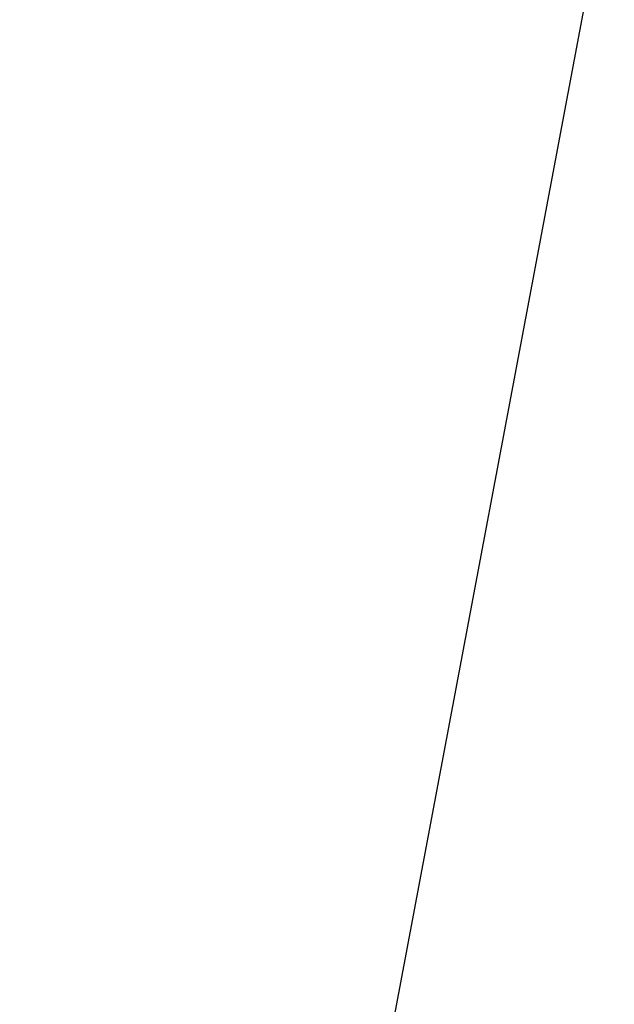
# Model space of a CAD drawing. Units: inches. Extents: x 3590 to 5167, y 65 to 1917.
# Tile 83 of 100: x 5051.4139 to 5051.5399, y 1788.6144 to 1788.8231. Entities that reach past the tile are written whole.
import ezdxf

# ---------------------------------------------------------------- set-up
doc = ezdxf.new("R2010")
doc.units = ezdxf.units.IN
for name, color, linetype, lineweight in [('A-ANNO-DIMS', 2, 'Continuous', 18), ('A-FLOR-PATT', 8, 'Continuous', 13), ('L-PLNT', 94, 'Continuous', 18)]:
    doc.layers.add(name, color=color, linetype=linetype, lineweight=lineweight)
doc.layers.add('DIENHOA', color=3, linetype='Continuous')
doc.styles.get("Standard").update_dxf_attribs({"font": 'arial.ttf'})
doc.dimstyles.new('ISO-25', dxfattribs={"dimtxt": 9, "dimasz": 2.5, "dimexe": 1.25, "dimexo": 0.625, "dimtad": 1, "dimdec": 1, "dimlunit": 3, "dimtxsty": 'Standard', "dimcen": 2.5, "dimadec": 0, "dimazin": 0, "dimtfac": 1, "dimtdec": 1, "dimtmove": 0, "dimatfit": 3, "dimfxl": 1, "dimarcsym": 0})

# ---------------------------------------------------------------- blocks, each defined once
blk = doc.blocks.new('Cay03_mb')
at = {"layer": 'DIENHOA'}
blk.add_lwpolyline([(87.9153, 628.5249), (75.4561, 544.1788), (61.2665, 461.1547), (46.1288, 379.1401), (30.8256, 297.8222), (16.1394, 216.8885), (2.8527, 136.0262), (-8.252, 54.9228), (-16.3923, -26.7346)], dxfattribs=at)
blk = doc.blocks.new('*D323')
at = {"layer": 'A-ANNO-DIMS', "color": 0, "lineweight": -2, "transparency": 16777216}
for p, q in [((5069.17227, 1795.21603), (5069.17227, 1874.95034)), ((5065.43703, 1795.21603), (5070.42227, 1795.21603)), ((5069.17227, 1769.30924), (5069.17227, 1792.71603)), ((5065.43703, 1766.80924), (5070.42227, 1766.80924))]:
    blk.add_line(p, q, dxfattribs=at)
at = {"layer": 'A-ANNO-DIMS', "color": 0, "transparency": 16777216}
for points in [[(5068.75561, 1792.71603), (5069.58894, 1792.71603), (5069.17227, 1795.21603)], [(5068.75561, 1769.30924), (5069.58894, 1769.30924), (5069.17227, 1766.80924)]]:
    blk.add_solid(points, dxfattribs=at)
at = {"layer": 'Defpoints', "color": 0, "transparency": 16777216}
for p in [(5064.81203, 1795.21603), (5069.17227, 1795.21603), (5064.81203, 1766.80924)]:
    blk.add_point(p, dxfattribs=at)
at = {"layer": 'A-ANNO-DIMS', "color": 0, "transparency": 16777216, "insert": (5063.89379, 1836.33318), "char_height": 9, "attachment_point": 5, "rotation": 90}
blk.add_mtext('2\'-4 1/2" TYP.', dxfattribs=at)

msp = doc.modelspace()

# ---------------------------------------------------------------- hatches: boundary and pattern name
at = {"layer": 'A-FLOR-PATT', "transparency": 33554687}
h = msp.add_hatch(dxfattribs=at)
h.set_pattern_fill('AR-HBONE', color=256, scale=0.2)
h.set_pattern_definition([(45, (-588.972, 0), (0, 28.73682), [60.96, -20.32]), (135, (-574.604, 14.368), (3e-15, 28.73682), [60.96, -20.32])])
h.paths.add_polyline_path([(5071.27403, 1796.99898), (4933.27403, 1796.99898), (4933.27403, 1753.99898), (4962.77403, 1753.99898, -0.414214), (4928.77403, 1719.99898), (4933.27403, 1718.99898), (4933.27403, 1334.99898), (5071.27403, 1334.99898)])
h.paths.add_polyline_path([(4951.78002, 1521.0767), (4951.7151, 1521.0404), (4951.56345, 1520.89532)], flags=16)
h.paths.add_polyline_path([(4952.267, 1521.37645), (4952.1977, 1521.37111), (4952.19823, 1521.35558)], flags=0)
h.paths.add_polyline_path([(4967.05076, 1529.72832), (4965.23122, 1528.69444), (4963.41109, 1527.71401), (4961.75649, 1526.85081), (4963.58887, 1527.44938), (4964.03555, 1527.47802), (4962.9755, 1527.24902), (4961.76022, 1526.85203), (4959.79219, 1525.83406), (4958.00498, 1524.89483), (4956.24031, 1523.92961), (4954.50395, 1522.91854), (4954.1294, 1522.68163), (4953.36051, 1521.99688), (4953.36558, 1521.99754), (4953.605, 1522.06367), (4955.10605, 1522.76083), (4956.92108, 1523.43405), (4958.67784, 1523.91513), (4960.35834, 1524.20036), (4961.94456, 1524.28606), (4964.17144, 1524.10849), (4965.95752, 1523.30903), (4963.86273, 1522.97565), (4965.18742, 1522.49898), (4963.36614, 1522.49715), (4961.54526, 1522.48682), (4959.76359, 1522.46077), (4958.30414, 1522.4188), (4957.97356, 1522.38829), (4956.30692, 1522.2324), (4954.71821, 1522.07143), (4953.25077, 1521.89915), (4953.52509, 1521.62277), (4954.33087, 1521.37883), (4956.24263, 1521.22987), (4958.03913, 1520.92952), (4959.68424, 1520.48339), (4961.16007, 1519.89569), (4963.10699, 1518.80022), (4964.39286, 1517.32518), (4962.97306, 1517.72596), (4964.55841, 1516.66059), (4965.40664, 1515.70779), (4963.50733, 1516.32179), (4961.67995, 1517.0051), (4959.93478, 1517.74489), (4958.2821, 1518.52833), (4956.73216, 1519.34257), (4955.29527, 1520.17478), (4954.67155, 1520.57237), (4954.51279, 1520.6271), (4955.65848, 1519.31837), (4956.70263, 1517.98232), (4957.64403, 1516.64663), (4958.48545, 1515.33439), (4959.54998, 1513.52398), (4960.43768, 1511.76936), (4958.84107, 1513.6196), (4957.45175, 1515.3249), (4955.8186, 1517.45855), (4956.66537, 1515.44764), (4957.11109, 1513.92292), (4957.44681, 1511.71434), (4957.07641, 1509.79288), (4956.53757, 1511.1103), (4955.99231, 1512.56892), (4955.44448, 1514.12509), (4954.89794, 1515.73518), (4954.35653, 1517.35553), (4953.82412, 1518.94251), (4953.30455, 1520.45247), (4953.06452, 1521.11563), (4952.97143, 1521.14607), (4952.94932, 1521.08646), (4952.72981, 1520.19905), (4953.3698, 1518.02364), (4953.75708, 1516.37279), (4954.05124, 1514.76538), (4954.26449, 1513.22121), (4954.47124, 1511.13121), (4954.4971, 1510.40174), (4954.40903, 1511.76006), (4954.26449, 1513.22121), (4954.05124, 1514.76538), (4953.75708, 1516.37279), (4953.3698, 1518.02364), (4952.87718, 1519.69813), (4952.7161, 1520.1412), (4952.53301, 1519.05871), (4952.37428, 1517.78881), (4952.21925, 1516.31167), (4952.04598, 1514.59986), (4951.83253, 1512.62598), (4951.55697, 1510.36259), (4951.20331, 1512.16818), (4950.85168, 1514.33931), (4950.98529, 1516.37594), (4951.6596, 1518.28625), (4952.59261, 1520.48085), (4952.35664, 1521.1299), (4951.85502, 1520.32753), (4950.83901, 1518.90828), (4949.77675, 1517.58658), (4948.91554, 1516.61731), (4948.11099, 1515.2561), (4947.0891, 1513.55389), (4945.88937, 1511.61495), (4946.32587, 1513.40232), (4946.5624, 1514.24913), (4945.52771, 1513.32668), (4944.58105, 1512.53126), (4946.01774, 1514.50825), (4947.2044, 1516.04763), (4947.89331, 1517.31331), (4949.30686, 1518.76446), (4950.41417, 1519.76716), (4950.45131, 1519.80628), (4952.267, 1521.37645), (4951.64457, 1521.49317), (4950.40371, 1521.17954), (4948.04447, 1520.35868), (4946.11863, 1519.45198), (4944.57182, 1518.47484), (4943.34962, 1517.44265), (4941.99695, 1515.91971), (4941.66146, 1515.27475), (4942.81332, 1516.98973), (4944.57182, 1518.47484), (4946.11863, 1519.45198), (4948.04447, 1520.35868), (4950.40371, 1521.17954), (4951.64457, 1521.49317), (4949.64678, 1521.86781), (4948.59979, 1521.75633), (4947.12629, 1521.5699), (4945.42015, 1521.34763), (4943.44969, 1521.10462), (4941.18319, 1520.85596), (4942.86028, 1521.61265), (4943.87308, 1522.03014), (4942.95216, 1521.9093), (4941.40968, 1521.48512), (4939.54287, 1520.67019), (4938.96775, 1520.2255), (4940.73284, 1521.29899), (4942.95216, 1521.9093), (4943.70184, 1522.00767), (4945.89419, 1522.69998), (4947.56488, 1522.71399), (4948.92086, 1522.56573), (4951.13144, 1522.18271), (4950.97062, 1522.2969), (4948.12924, 1523.00563), (4946.03496, 1523.70671), (4944.23235, 1524.52143), (4942.70692, 1525.46111), (4941.44419, 1526.53707), (4940.42968, 1527.76062), (4939.6489, 1529.14306), (4941.42091, 1528.12232), (4943.14742, 1527.13248), (4944.84093, 1526.17457), (4946.51394, 1525.24959), (4948.17893, 1524.35855), (4948.36457, 1524.26336), (4946.47531, 1526.04459), (4945.18083, 1527.54042), (4944.19039, 1529.03339), (4943.49559, 1530.53985), (4943.27808, 1531.3597), (4942.49849, 1531.91903), (4943.11353, 1531.76249), (4942.95927, 1533.6586), (4944.13953, 1531.9886), (4944.61171, 1531.32339), (4946.20163, 1530.46341), (4947.48567, 1529.50925), (4948.79027, 1528.22649), (4950.36754, 1526.23746), (4949.48547, 1528.15549), (4948.85128, 1530.12254), (4948.49054, 1532.04127), (4948.38105, 1533.91822), (4948.50062, 1535.7599), (4948.82704, 1537.57284), (4949.41803, 1535.56526), (4949.95684, 1533.56932), (4950.46414, 1531.5861), (4950.96058, 1529.6167), (4951.3911, 1527.95448), (4951.72352, 1530.68689), (4952.20106, 1532.57994), (4952.88914, 1534.32964), (4953.77035, 1535.95123), (4954.82726, 1537.45995), (4954.52145, 1535.38966), (4954.27314, 1533.93684), (4955.57999, 1535.6627), (4956.74758, 1536.73859), (4956.15852, 1534.78029), (4955.58917, 1532.87334), (4955.04336, 1531.00581), (4954.52493, 1529.16576), (4954.03771, 1527.34127), (4953.63833, 1525.73298), (4953.61143, 1525.58564), (4953.39805, 1524.16565), (4953.38219, 1524.00887), (4954.06955, 1525.47563), (4954.91212, 1527.02173), (4956.13627, 1528.89351), (4957.84668, 1530.57701), (4959.37601, 1531.54014), (4958.25596, 1530.10398), (4957.14284, 1528.66291), (4956.06626, 1527.24305), (4955.05579, 1525.87054), (4954.14104, 1524.57149), (4953.35159, 1523.37204), (4953.31079, 1523.30299), (4953.27253, 1522.92478), (4953.26102, 1522.38213), (4954.1031, 1523.37273), (4954.63005, 1524.28376), (4955.96149, 1526.35767), (4957.23002, 1528.12969), (4958.42057, 1529.60864), (4960.03671, 1531.36792), (4961.3736, 1532.3752), (4962.1015, 1532.77), (4961.06994, 1531.06113), (4959.98733, 1529.43811), (4958.86851, 1527.90803), (4958.15046, 1527.00742), (4959.80291, 1528.00314), (4961.58854, 1528.79257), (4963.39087, 1529.32783), (4965.21118, 1529.63205)], flags=16)
h.paths.add_polyline_path([(4962.94387, 1523.18187), (4961.10714, 1523.42192), (4960.39205, 1523.36158), (4962.34964, 1523.33061)], flags=0)
h.paths.add_polyline_path([(5049.54129, 1584.55089), (5049.47636, 1584.51458), (5049.32471, 1584.3695)], flags=16)
h.paths.add_polyline_path([(5050.02827, 1584.85063), (5049.95897, 1584.84529), (5049.95949, 1584.82976)], flags=0)
h.paths.add_polyline_path([(5042.33308, 1581.94902), (5043.8799, 1582.92616), (5045.80573, 1583.83286), (5048.16498, 1584.65372), (5049.40583, 1584.96736), (5047.40804, 1585.34199), (5046.36106, 1585.23052), (5044.88755, 1585.04408), (5043.18142, 1584.82181), (5041.21095, 1584.5788), (5038.94446, 1584.33014), (5040.62155, 1585.08683), (5041.63434, 1585.50432), (5040.71343, 1585.38348), (5039.17095, 1584.9593), (5037.30414, 1584.14438), (5036.72901, 1583.69969), (5038.4941, 1584.77317), (5040.71343, 1585.38348), (5041.4631, 1585.48185), (5043.65545, 1586.17416), (5045.32615, 1586.18818), (5046.68212, 1586.03992), (5048.8927, 1585.6569), (5048.73188, 1585.77108), (5045.89051, 1586.47981), (5043.79622, 1587.18089), (5041.99361, 1587.99561), (5040.46818, 1588.9353), (5039.20546, 1590.01125), (5038.19095, 1591.2348), (5037.41016, 1592.61725), (5039.18217, 1591.5965), (5040.90868, 1590.60667), (5042.6022, 1589.64876), (5044.2752, 1588.72378), (5045.94019, 1587.83274), (5046.12584, 1587.73754), (5044.23658, 1589.51878), (5042.9421, 1591.01461), (5041.95166, 1592.50757), (5041.25685, 1594.01403), (5041.03935, 1594.83388), (5040.25976, 1595.39321), (5040.8748, 1595.23667), (5040.72054, 1597.13279), (5041.9008, 1595.46278), (5042.37297, 1594.79758), (5043.96289, 1593.93759), (5045.24694, 1592.98344), (5046.55153, 1591.70068), (5048.12881, 1589.71164), (5047.24673, 1591.62967), (5046.61254, 1593.59672), (5046.2518, 1595.51546), (5046.14232, 1597.3924), (5046.26189, 1599.23408), (5046.5883, 1601.04703), (5047.17929, 1599.03944), (5047.71811, 1597.0435), (5048.22541, 1595.06028), (5048.72184, 1593.09089), (5049.15237, 1591.42866), (5049.48478, 1594.16107), (5049.96233, 1596.05412), (5050.65041, 1597.80382), (5051.53161, 1599.42541), (5052.58852, 1600.93414), (5052.28271, 1598.86384), (5052.03441, 1597.41102), (5053.34126, 1599.13689), (5054.50884, 1600.21277), (5053.91979, 1598.25447), (5053.35044, 1596.34752), (5052.80463, 1594.47999), (5052.2862, 1592.63995), (5051.79898, 1590.81546), (5051.39959, 1589.20716), (5051.3727, 1589.05983), (5051.15931, 1587.63984), (5051.14346, 1587.48305), (5051.83082, 1588.94982), (5052.67339, 1590.49592), (5053.89754, 1592.3677), (5055.60794, 1594.05119), (5057.13728, 1595.01432), (5056.01722, 1593.57817), (5054.90411, 1592.1371), (5053.82752, 1590.71724), (5052.81705, 1589.34472), (5051.9023, 1588.04567), (5051.11286, 1586.84622), (5051.07205, 1586.77718), (5051.03379, 1586.39896), (5051.02228, 1585.85631), (5051.86437, 1586.84692), (5052.39131, 1587.75794), (5053.72275, 1589.83185), (5054.99128, 1591.60387), (5056.18183, 1593.08282), (5057.79798, 1594.84211), (5059.13486, 1595.84938), (5059.86276, 1596.24419), (5058.83121, 1594.53531), (5057.7486, 1592.9123), (5056.62978, 1591.38221), (5055.91173, 1590.4816), (5057.56418, 1591.47732), (5059.34981, 1592.26675), (5061.15214, 1592.80202), (5062.97245, 1593.10624), (5064.81203, 1593.20251), (5062.99248, 1592.16863), (5061.17235, 1591.18819), (5059.51775, 1590.325), (5061.35014, 1590.92356), (5061.79682, 1590.95221), (5060.73676, 1590.7232), (5059.52148, 1590.32622), (5057.55345, 1589.30825), (5055.76625, 1588.36901), (5054.00157, 1587.40379), (5052.26521, 1586.39273), (5051.89067, 1586.15581), (5051.12177, 1585.47106), (5051.12684, 1585.47172), (5051.36627, 1585.53786), (5052.86732, 1586.23502), (5054.68234, 1586.90824), (5056.4391, 1587.38931), (5058.1196, 1587.67454), (5059.70582, 1587.76024), (5061.93271, 1587.58268), (5063.71878, 1586.78321), (5061.62399, 1586.44983), (5062.94869, 1585.97317), (5061.12741, 1585.97133), (5059.30653, 1585.961), (5057.52486, 1585.93496), (5056.06541, 1585.89299), (5055.73482, 1585.86247), (5054.06819, 1585.70658), (5052.47947, 1585.54561), (5051.01204, 1585.37333), (5051.28635, 1585.09695), (5052.09214, 1584.85301), (5054.00389, 1584.70406), (5055.8004, 1584.4037), (5057.44551, 1583.95757), (5058.92133, 1583.36987), (5060.86825, 1582.27441), (5062.15413, 1580.79937), (5060.73433, 1581.20015), (5062.31967, 1580.13477), (5063.1679, 1579.18198), (5061.2686, 1579.79597), (5059.44122, 1580.47928), (5057.69605, 1581.21908), (5056.04336, 1582.00251), (5054.49343, 1582.81675), (5053.05653, 1583.64897), (5052.43281, 1584.04656), (5052.27405, 1584.10128), (5053.41974, 1582.79255), (5054.4639, 1581.4565), (5055.40529, 1580.12081), (5056.24672, 1578.80858), (5057.31125, 1576.99816), (5058.19895, 1575.24354), (5056.60234, 1577.09378), (5055.21301, 1578.79908), (5053.57987, 1580.93274), (5054.42664, 1578.92183), (5054.87235, 1577.3971), (5055.20808, 1575.18852), (5054.83767, 1573.26706), (5054.29883, 1574.58448), (5053.75357, 1576.0431), (5053.20575, 1577.59927), (5052.6592, 1579.20936), (5052.1178, 1580.82971), (5051.58538, 1582.41669), (5051.06582, 1583.92666), (5050.82578, 1584.58981), (5050.7327, 1584.62025), (5050.71058, 1584.56064), (5050.49108, 1583.67323), (5051.13107, 1581.49782), (5051.51835, 1579.84698), (5051.8125, 1578.23957), (5052.02575, 1576.69539), (5052.23251, 1574.6054), (5052.25836, 1573.87593), (5052.1703, 1575.23424), (5052.02575, 1576.69539), (5051.8125, 1578.23957), (5051.51835, 1579.84698), (5051.13107, 1581.49782), (5050.63844, 1583.17231), (5050.47736, 1583.61538), (5050.29428, 1582.53289), (5050.13554, 1581.26299), (5049.98051, 1579.78585), (5049.80724, 1578.07405), (5049.59379, 1576.10016), (5049.31823, 1573.83678), (5048.96458, 1575.64237), (5048.61294, 1577.8135), (5048.74656, 1579.85012), (5049.42086, 1581.76043), (5050.35388, 1583.95503), (5050.1179, 1584.60408), (5049.61629, 1583.80172), (5048.60027, 1582.38246), (5047.53801, 1581.06076), (5046.67681, 1580.09149), (5045.87225, 1578.73029), (5044.85036, 1577.02808), (5043.65063, 1575.08913), (5044.08713, 1576.8765), (5044.32366, 1577.72331), (5043.28898, 1576.80086), (5042.34232, 1576.00545), (5043.779, 1577.98243), (5044.96566, 1579.52182), (5045.65457, 1580.78749), (5047.06813, 1582.23865), (5048.17543, 1583.24134), (5048.21258, 1583.28047), (5050.02827, 1584.85063), (5049.40583, 1584.96736), (5048.16498, 1584.65372), (5045.80573, 1583.83286), (5043.8799, 1582.92616), (5042.33308, 1581.94902), (5041.11088, 1580.91684), (5039.75821, 1579.39389), (5039.42272, 1578.74894), (5040.57458, 1580.46391)], flags=16)
h.paths.add_polyline_path([(4954.79872, 1533.12029), (4954.26249, 1532.07935), (4953.83112, 1530.93464), (4953.50472, 1529.63602), (4953.28338, 1528.13331), (4953.16721, 1526.37637), (4953.15631, 1524.31504), (4953.27669, 1521.23629), (4952.80168, 1521.84177), (4951.55695, 1521.99789), (4950.97575, 1521.9613), (4952.66059, 1521.94097), (4952.80168, 1521.84177), (4953.15249, 1523.59258), (4953.16721, 1526.37637), (4953.28338, 1528.13331), (4953.60929, 1530.34598), (4954.45558, 1532.59174)], flags=0)
h.paths.add_polyline_path([(5050.56294, 1585.31596), (5049.31822, 1585.47208), (5048.73702, 1585.43548), (5050.42186, 1585.41516), (5050.56294, 1585.31596), (5050.91375, 1587.06676), (5050.92848, 1589.85056), (5051.04465, 1591.6075), (5051.37055, 1593.82017), (5052.21684, 1596.06593), (5052.55999, 1596.59447), (5052.02375, 1595.55353), (5051.59238, 1594.40883), (5051.26598, 1593.1102), (5051.04465, 1591.6075), (5050.92848, 1589.85056), (5050.91757, 1587.78922), (5051.03795, 1584.71048)], flags=0)
h.paths.add_polyline_path([(5058.15332, 1586.83576), (5060.11091, 1586.80479), (5060.70514, 1586.65605), (5058.8684, 1586.8961)], flags=0)
h.paths.add_polyline_path([(5049.54129, 1430.93611), (5049.47636, 1430.8998), (5049.32471, 1430.75472)], flags=16)
h.paths.add_polyline_path([(5050.02827, 1431.23585), (5049.95897, 1431.23051), (5049.95949, 1431.21498)], flags=0)
h.paths.add_polyline_path([(5046.5883, 1447.43225), (5047.17929, 1445.42467), (5047.71811, 1443.42872), (5048.22541, 1441.4455), (5048.72184, 1439.47611), (5049.15237, 1437.81388), (5049.48478, 1440.5463), (5049.96233, 1442.43934), (5050.65041, 1444.18904), (5051.53161, 1445.81063), (5052.58852, 1447.31936), (5052.28271, 1445.24906), (5052.03441, 1443.79624), (5053.34126, 1445.52211), (5054.50884, 1446.59799), (5053.91979, 1444.63969), (5053.35044, 1442.73274), (5052.80463, 1440.86521), (5052.2862, 1439.02517), (5051.79898, 1437.20068), (5051.39959, 1435.59238), (5051.3727, 1435.44505), (5051.15931, 1434.02506), (5051.14346, 1433.86828), (5051.83082, 1435.33504), (5052.67339, 1436.88114), (5053.89754, 1438.75292), (5055.60794, 1440.43641), (5057.13728, 1441.39954), (5056.01722, 1439.96339), (5054.90411, 1438.52232), (5053.82752, 1437.10246), (5052.81705, 1435.72994), (5051.9023, 1434.4309), (5051.11286, 1433.23145), (5051.07205, 1433.1624), (5051.03379, 1432.78418), (5051.02228, 1432.24153), (5051.86437, 1433.23214), (5052.39131, 1434.14316), (5053.72275, 1436.21707), (5054.99128, 1437.98909), (5056.18183, 1439.46805), (5057.79798, 1441.22733), (5059.13486, 1442.23461), (5059.86276, 1442.62941), (5058.83121, 1440.92053), (5057.7486, 1439.29752), (5056.62978, 1437.76743), (5055.91173, 1436.86682), (5057.56418, 1437.86255), (5059.34981, 1438.65197), (5061.15214, 1439.18724), (5062.97245, 1439.49146), (5064.81203, 1439.58773), (5062.99248, 1438.55385), (5061.17235, 1437.57342), (5059.51775, 1436.71022), (5061.35014, 1437.30879), (5061.79682, 1437.33743), (5060.73676, 1437.10842), (5059.52148, 1436.71144), (5057.55345, 1435.69347), (5055.76625, 1434.75423), (5054.00157, 1433.78901), (5052.26521, 1432.77795), (5051.89067, 1432.54103), (5051.12177, 1431.85628), (5051.12684, 1431.85694), (5051.36627, 1431.92308), (5052.86732, 1432.62024), (5054.68234, 1433.29346), (5056.4391, 1433.77453), (5058.1196, 1434.05976), (5059.70582, 1434.14546), (5061.93271, 1433.9679), (5063.71878, 1433.16843), (5061.62399, 1432.83505), (5062.94869, 1432.35839), (5061.12741, 1432.35655), (5059.30653, 1432.34623), (5057.52486, 1432.32018), (5056.06541, 1432.27821), (5055.73482, 1432.24769), (5054.06819, 1432.09181), (5052.47947, 1431.93083), (5051.01204, 1431.75856), (5051.28635, 1431.48218), (5052.09214, 1431.23823), (5054.00389, 1431.08928), (5055.8004, 1430.78892), (5057.44551, 1430.34279), (5058.92133, 1429.75509), (5060.86825, 1428.65963), (5062.15413, 1427.18459), (5060.73433, 1427.58537), (5062.31967, 1426.52), (5063.1679, 1425.5672), (5061.2686, 1426.18119), (5059.44122, 1426.86451), (5057.69605, 1427.6043), (5056.04336, 1428.38773), (5054.49343, 1429.20197), (5053.05653, 1430.03419), (5052.43281, 1430.43178), (5052.27405, 1430.48651), (5053.41974, 1429.17777), (5054.4639, 1427.84172), (5055.40529, 1426.50603), (5056.24672, 1425.1938), (5057.31125, 1423.38338), (5058.19895, 1421.62877), (5056.60234, 1423.479), (5055.21301, 1425.1843), (5053.57987, 1427.31796), (5054.42664, 1425.30705), (5054.87235, 1423.78233), (5055.20808, 1421.57374), (5054.83767, 1419.65228), (5054.29883, 1420.9697), (5053.75357, 1422.42832), (5053.20575, 1423.9845), (5052.6592, 1425.59458), (5052.1178, 1427.21493), (5051.58538, 1428.80191), (5051.06582, 1430.31188), (5050.82578, 1430.97503), (5050.7327, 1431.00547), (5050.71058, 1430.94586), (5050.49108, 1430.05845), (5051.13107, 1427.88305), (5051.51835, 1426.2322), (5051.8125, 1424.62479), (5052.02575, 1423.08061), (5052.23251, 1420.99062), (5052.25836, 1420.26115), (5052.1703, 1421.61947), (5052.02575, 1423.08061), (5051.8125, 1424.62479), (5051.51835, 1426.2322), (5051.13107, 1427.88305), (5050.63844, 1429.55753), (5050.47736, 1430.0006), (5050.29428, 1428.91811), (5050.13554, 1427.64821), (5049.98051, 1426.17107), (5049.80724, 1424.45927), (5049.59379, 1422.48539), (5049.31823, 1420.222), (5048.96458, 1422.02759), (5048.61294, 1424.19872), (5048.74656, 1426.23534), (5049.42086, 1428.14565), (5050.35388, 1430.34025), (5050.1179, 1430.98931), (5049.61629, 1430.18694), (5048.60027, 1428.76768), (5047.53801, 1427.44598), (5046.67681, 1426.47671), (5045.87225, 1425.11551), (5044.85036, 1423.4133), (5043.65063, 1421.47435), (5044.08713, 1423.26172), (5044.32366, 1424.10854), (5043.28898, 1423.18608), (5042.34232, 1422.39067), (5043.779, 1424.36765), (5044.96566, 1425.90704), (5045.65457, 1427.17272), (5047.06813, 1428.62387), (5048.17543, 1429.62657), (5048.21258, 1429.66569), (5050.02827, 1431.23585), (5049.40583, 1431.35258), (5048.16498, 1431.03894), (5045.80573, 1430.21809), (5043.8799, 1429.31139), (5042.33308, 1428.33424), (5041.11088, 1427.30206), (5039.75821, 1425.77911), (5039.42272, 1425.13416), (5040.57458, 1426.84914), (5042.33308, 1428.33424), (5043.8799, 1429.31139), (5045.80573, 1430.21809), (5048.16498, 1431.03894), (5049.40583, 1431.35258), (5047.40804, 1431.72722), (5046.36106, 1431.61574), (5044.88755, 1431.42931), (5043.18142, 1431.20704), (5041.21095, 1430.96402), (5038.94446, 1430.71536), (5040.62155, 1431.47205), (5041.63434, 1431.88954), (5040.71343, 1431.76871), (5039.17095, 1431.34453), (5037.30414, 1430.5296), (5036.72901, 1430.08491), (5038.4941, 1431.1584), (5040.71343, 1431.76871), (5041.4631, 1431.86707), (5043.65545, 1432.55939), (5045.32615, 1432.5734), (5046.68212, 1432.42514), (5048.8927, 1432.04212), (5048.73188, 1432.1563), (5045.89051, 1432.86503), (5043.79622, 1433.56611), (5041.99361, 1434.38083), (5040.46818, 1435.32052), (5039.20546, 1436.39648), (5038.19095, 1437.62002), (5037.41016, 1439.00247), (5039.18217, 1437.98172), (5040.90868, 1436.99189), (5042.6022, 1436.03398), (5044.2752, 1435.109), (5045.94019, 1434.21796), (5046.12584, 1434.12276), (5044.23658, 1435.904), (5042.9421, 1437.39983), (5041.95166, 1438.8928), (5041.25685, 1440.39925), (5041.03935, 1441.2191), (5040.25976, 1441.77844), (5040.8748, 1441.62189), (5040.72054, 1443.51801), (5041.9008, 1441.848), (5042.37297, 1441.1828), (5043.96289, 1440.32282), (5045.24694, 1439.36866), (5046.55153, 1438.0859), (5048.12881, 1436.09686), (5047.24673, 1438.01489), (5046.61254, 1439.98195), (5046.2518, 1441.90068), (5046.14232, 1443.77762), (5046.26189, 1445.6193)], flags=16)
h.paths.add_polyline_path([(5052.38176, 1444.25496), (5051.62263, 1442.77987), (5052.02375, 1441.93875), (5052.55999, 1442.9797)], flags=0)
h.paths.add_polyline_path([(5050.56294, 1431.70118), (5049.31822, 1431.8573), (5048.73702, 1431.82071), (5050.42186, 1431.80038)], flags=0)
h.paths.add_polyline_path([(5058.15332, 1433.22098), (5060.11091, 1433.19001), (5060.70514, 1433.04127), (5058.8684, 1433.28132)], flags=0)
h.paths.add_polyline_path([(5049.54129, 1352.28535), (5049.47636, 1352.24904), (5049.32471, 1352.10396)], flags=16)
h.paths.add_polyline_path([(5050.02827, 1352.58509), (5049.95897, 1352.57975), (5049.95949, 1352.56422)], flags=0)
h.paths.add_polyline_path([(5046.5883, 1368.78149), (5047.17929, 1366.7739), (5047.71811, 1364.77796), (5048.22541, 1362.79474), (5048.72184, 1360.82534), (5049.15237, 1359.16312), (5049.48478, 1361.89553), (5049.96233, 1363.78858), (5050.65041, 1365.53828), (5051.53161, 1367.15987), (5052.58852, 1368.6686), (5052.28271, 1366.5983), (5052.03441, 1365.14548), (5053.34126, 1366.87135), (5054.50884, 1367.94723), (5053.91979, 1365.98893), (5053.35044, 1364.08198), (5052.80463, 1362.21445), (5052.2862, 1360.37441), (5051.79898, 1358.54992), (5051.39959, 1356.94162), (5051.3727, 1356.79428), (5051.15931, 1355.37429), (5051.14346, 1355.21751), (5051.83082, 1356.68428), (5052.67339, 1358.23037), (5053.89754, 1360.10216), (5055.60794, 1361.78565), (5057.13728, 1362.74878), (5056.01722, 1361.31262), (5054.90411, 1359.87155), (5053.82752, 1358.4517), (5052.81705, 1357.07918), (5051.9023, 1355.78013), (5051.11286, 1354.58068), (5051.07205, 1354.51164), (5051.03379, 1354.13342), (5051.02228, 1353.59077), (5051.86437, 1354.58137), (5052.39131, 1355.4924), (5053.72275, 1357.56631), (5054.99128, 1359.33833), (5056.18183, 1360.81728), (5057.79798, 1362.57656), (5059.13486, 1363.58384), (5059.86276, 1363.97864), (5058.83121, 1362.26977), (5057.7486, 1360.64675), (5056.62978, 1359.11667), (5055.91173, 1358.21606), (5057.56418, 1359.21178), (5059.34981, 1360.00121), (5061.15214, 1360.53648), (5062.97245, 1360.84069), (5064.81203, 1360.93697), (5062.99248, 1359.90308), (5061.17235, 1358.92265), (5059.51775, 1358.05946), (5061.35014, 1358.65802), (5061.79682, 1358.68666), (5060.73676, 1358.45766), (5059.52148, 1358.06068), (5057.55345, 1357.0427), (5055.76625, 1356.10347), (5054.00157, 1355.13825), (5052.26521, 1354.12718), (5051.89067, 1353.89027), (5051.12177, 1353.20552), (5051.12684, 1353.20618), (5051.36627, 1353.27231), (5052.86732, 1353.96947), (5054.68234, 1354.6427), (5056.4391, 1355.12377), (5058.1196, 1355.409), (5059.70582, 1355.4947), (5061.93271, 1355.31713), (5063.71878, 1354.51767), (5061.62399, 1354.18429), (5062.94869, 1353.70763), (5061.12741, 1353.70579), (5059.30653, 1353.69546), (5057.52486, 1353.66942), (5056.06541, 1353.62744), (5055.73482, 1353.59693), (5054.06819, 1353.44104), (5052.47947, 1353.28007), (5051.01204, 1353.10779), (5051.28635, 1352.83141), (5052.09214, 1352.58747), (5054.00389, 1352.43852), (5055.8004, 1352.13816), (5057.44551, 1351.69203), (5058.92133, 1351.10433), (5060.86825, 1350.00887), (5062.15413, 1348.53382), (5060.73433, 1348.9346), (5062.31967, 1347.86923), (5063.1679, 1346.91643), (5061.2686, 1347.53043), (5059.44122, 1348.21374), (5057.69605, 1348.95353), (5056.04336, 1349.73697), (5054.49343, 1350.55121), (5053.05653, 1351.38342), (5052.43281, 1351.78101), (5052.27405, 1351.83574), (5053.41974, 1350.52701), (5054.4639, 1349.19096), (5055.40529, 1347.85527), (5056.24672, 1346.54303), (5057.31125, 1344.73262), (5058.19895, 1342.978), (5056.60234, 1344.82824), (5055.21301, 1346.53354), (5053.57987, 1348.6672), (5054.42664, 1346.65629), (5054.87235, 1345.13156), (5055.20808, 1342.92298), (5054.83767, 1341.00152), (5054.29883, 1342.31894), (5053.75357, 1343.77756), (5053.20575, 1345.33373), (5052.6592, 1346.94382), (5052.1178, 1348.56417), (5051.58538, 1350.15115), (5051.06582, 1351.66111), (5050.82578, 1352.32427), (5050.7327, 1352.35471), (5050.71058, 1352.2951), (5050.49108, 1351.40769), (5051.13107, 1349.23228), (5051.51835, 1347.58144), (5051.8125, 1345.97403), (5052.02575, 1344.42985), (5052.23251, 1342.33986), (5052.25836, 1341.61039), (5052.1703, 1342.9687), (5052.02575, 1344.42985), (5051.8125, 1345.97403), (5051.51835, 1347.58144), (5051.13107, 1349.23228), (5050.63844, 1350.90677), (5050.47736, 1351.34984), (5050.29428, 1350.26735), (5050.13554, 1348.99745), (5049.98051, 1347.52031), (5049.80724, 1345.80851), (5049.59379, 1343.83462), (5049.31823, 1341.57124), (5048.96458, 1343.37683), (5048.61294, 1345.54796), (5048.74656, 1347.58458), (5049.42086, 1349.49489), (5050.35388, 1351.68949), (5050.1179, 1352.33854), (5049.61629, 1351.53617), (5048.60027, 1350.11692), (5047.53801, 1348.79522), (5046.67681, 1347.82595), (5045.87225, 1346.46475), (5044.85036, 1344.76253), (5043.65063, 1342.82359), (5044.08713, 1344.61096), (5044.32366, 1345.45777), (5043.28898, 1344.53532), (5042.34232, 1343.7399), (5043.779, 1345.71689), (5044.96566, 1347.25627), (5045.65457, 1348.52195), (5047.06813, 1349.9731), (5048.17543, 1350.9758), (5048.21258, 1351.01493), (5050.02827, 1352.58509), (5049.40583, 1352.70181), (5048.16498, 1352.38818), (5045.80573, 1351.56732), (5043.8799, 1350.66062), (5042.33308, 1349.68348), (5041.11088, 1348.65129), (5039.75821, 1347.12835), (5039.42272, 1346.4834), (5040.57458, 1348.19837), (5042.33308, 1349.68348), (5043.8799, 1350.66062), (5045.80573, 1351.56732), (5048.16498, 1352.38818), (5049.40583, 1352.70181), (5047.40804, 1353.07645), (5046.36106, 1352.96498), (5044.88755, 1352.77854), (5043.18142, 1352.55627), (5041.21095, 1352.31326), (5038.94446, 1352.0646), (5040.62155, 1352.82129), (5041.63434, 1353.23878), (5040.71343, 1353.11794), (5039.17095, 1352.69376), (5037.30414, 1351.87884), (5036.72901, 1351.43415), (5038.4941, 1352.50763), (5040.71343, 1353.11794), (5041.4631, 1353.21631), (5043.65545, 1353.90862), (5045.32615, 1353.92263), (5046.68212, 1353.77438), (5048.8927, 1353.39136), (5048.73188, 1353.50554), (5045.89051, 1354.21427), (5043.79622, 1354.91535), (5041.99361, 1355.73007), (5040.46818, 1356.66975), (5039.20546, 1357.74571), (5038.19095, 1358.96926), (5037.41016, 1360.35171), (5039.18217, 1359.33096), (5040.90868, 1358.34112), (5042.6022, 1357.38321), (5044.2752, 1356.45824), (5045.94019, 1355.5672), (5046.12584, 1355.472), (5044.23658, 1357.25323), (5042.9421, 1358.74906), (5041.95166, 1360.24203), (5041.25685, 1361.74849), (5041.03935, 1362.56834), (5040.25976, 1363.12767), (5040.8748, 1362.97113), (5040.72054, 1364.86725), (5041.9008, 1363.19724), (5042.37297, 1362.53203), (5043.96289, 1361.67205), (5045.24694, 1360.7179), (5046.55153, 1359.43513), (5048.12881, 1357.4461), (5047.24673, 1359.36413), (5046.61254, 1361.33118), (5046.2518, 1363.24992), (5046.14232, 1365.12686), (5046.26189, 1366.96854)], flags=16)
h.paths.add_polyline_path([(5052.38176, 1365.6042), (5051.62263, 1364.12911), (5052.02375, 1363.28799), (5052.55999, 1364.32893)], flags=0)
h.paths.add_polyline_path([(4951.78002, 1698.04081), (4951.7151, 1698.0045), (4951.56345, 1697.85942)], flags=16)
h.paths.add_polyline_path([(4952.267, 1698.34055), (4952.1977, 1698.33521), (4952.19823, 1698.31968)], flags=0)
h.paths.add_polyline_path([(4957.07641, 1686.75698), (4956.53757, 1688.0744), (4955.99231, 1689.53302), (4955.44448, 1691.08919), (4954.89794, 1692.69928), (4954.35653, 1694.31963), (4953.82412, 1695.90661), (4953.30455, 1697.41658), (4953.06452, 1698.07973), (4952.97143, 1698.11017), (4952.94932, 1698.05056), (4952.72981, 1697.16315), (4953.3698, 1694.98774), (4953.75708, 1693.3369), (4954.05124, 1691.72949), (4954.26449, 1690.18531), (4954.47124, 1688.09532), (4954.4971, 1687.36585), (4954.40903, 1688.72416), (4954.26449, 1690.18531), (4954.05124, 1691.72949), (4953.75708, 1693.3369), (4953.3698, 1694.98774), (4952.87718, 1696.66223), (4952.7161, 1697.1053), (4952.53301, 1696.02281), (4952.37428, 1694.75291), (4952.21925, 1693.27577), (4952.04598, 1691.56397), (4951.83253, 1689.59008), (4951.55697, 1687.3267), (4951.20331, 1689.13229), (4950.85168, 1691.30342), (4950.98529, 1693.34004), (4951.6596, 1695.25035), (4952.59261, 1697.44495), (4952.35664, 1698.09401), (4951.85502, 1697.29164), (4950.83901, 1695.87238), (4949.77675, 1694.55068), (4948.91554, 1693.58141), (4948.11099, 1692.22021), (4947.0891, 1690.518), (4945.88937, 1688.57905), (4946.32587, 1690.36642), (4946.5624, 1691.21323), (4945.52771, 1690.29078), (4944.58105, 1689.49537), (4946.01774, 1691.47235), (4947.2044, 1693.01174), (4947.89331, 1694.27741), (4949.30686, 1695.72857), (4950.41417, 1696.73127), (4950.45131, 1696.77039), (4952.267, 1698.34055), (4951.64457, 1698.45728), (4950.40371, 1698.14364), (4948.04447, 1697.32278), (4946.11863, 1696.41608), (4944.57182, 1695.43894), (4943.34962, 1694.40676), (4941.99695, 1692.88381), (4941.66146, 1692.23886), (4942.81332, 1693.95383), (4944.57182, 1695.43894), (4946.11863, 1696.41608), (4948.04447, 1697.32278), (4950.40371, 1698.14364), (4951.64457, 1698.45728), (4949.64678, 1698.83191), (4948.59979, 1698.72044), (4947.12629, 1698.53401), (4945.42015, 1698.31174), (4943.44969, 1698.06872), (4941.18319, 1697.82006), (4942.86028, 1698.57675), (4943.87308, 1698.99424), (4942.95216, 1698.8734), (4941.40968, 1698.44922), (4939.54287, 1697.6343), (4938.96775, 1697.18961), (4940.73284, 1698.26309), (4942.95216, 1698.8734), (4943.70184, 1698.97177), (4945.89419, 1699.66409), (4947.56488, 1699.6781), (4948.92086, 1699.52984), (4951.13144, 1699.14682), (4950.97062, 1699.261), (4948.12924, 1699.96973), (4946.03496, 1700.67081), (4944.23235, 1701.48553), (4942.70692, 1702.42522), (4941.44419, 1703.50117), (4940.42968, 1704.72472), (4939.6489, 1706.10717), (4941.42091, 1705.08642), (4943.14742, 1704.09659), (4944.84093, 1703.13868), (4946.51394, 1702.2137), (4948.17893, 1701.32266), (4948.36457, 1701.22746), (4946.47531, 1703.0087), (4945.18083, 1704.50453), (4944.19039, 1705.9975), (4943.49559, 1707.50395), (4943.27808, 1708.3238), (4942.49849, 1708.88314), (4943.11353, 1708.72659), (4942.95927, 1710.62271), (4944.13953, 1708.9527), (4944.61171, 1708.2875), (4946.20163, 1707.42751), (4947.48567, 1706.47336), (4948.79027, 1705.1906), (4950.36754, 1703.20156), (4949.48547, 1705.11959), (4948.85128, 1707.08664), (4948.49054, 1709.00538), (4948.38105, 1710.88232), (4948.50062, 1712.724), (4948.82704, 1714.53695), (4949.41803, 1712.52937), (4949.95684, 1710.53342), (4950.46414, 1708.5502), (4950.96058, 1706.58081), (4951.3911, 1704.91858), (4951.72352, 1707.65099), (4952.20106, 1709.54404), (4952.88914, 1711.29374), (4953.77035, 1712.91533), (4954.82726, 1714.42406), (4954.52145, 1712.35376), (4954.27314, 1710.90094), (4955.57999, 1712.62681), (4956.74758, 1713.70269), (4956.15852, 1711.74439), (4955.58917, 1709.83744), (4955.04336, 1707.96991), (4954.52493, 1706.12987), (4954.03771, 1704.30538), (4953.63833, 1702.69708), (4953.61143, 1702.54975), (4953.39805, 1701.12976), (4953.38219, 1700.97297), (4954.06955, 1702.43974), (4954.91212, 1703.98584), (4956.13627, 1705.85762), (4957.84668, 1707.54111), (4959.37601, 1708.50424), (4958.25596, 1707.06809), (4957.14284, 1705.62702), (4956.06626, 1704.20716), (4955.05579, 1702.83464), (4954.14104, 1701.53559), (4953.35159, 1700.33614), (4953.31079, 1700.2671), (4953.27253, 1699.88888), (4953.26102, 1699.34623), (4954.1031, 1700.33684), (4954.63005, 1701.24786), (4955.96149, 1703.32177), (4957.23002, 1705.09379), (4958.42057, 1706.57274), (4960.03671, 1708.33203), (4961.3736, 1709.33931), (4962.1015, 1709.73411), (4961.06994, 1708.02523), (4959.98733, 1706.40222), (4958.86851, 1704.87213), (4958.15046, 1703.97152), (4959.80291, 1704.96725), (4961.58854, 1705.75667), (4963.39087, 1706.29194), (4965.21118, 1706.59616), (4967.05076, 1706.69243), (4965.23122, 1705.65855), (4963.41109, 1704.67811), (4961.75649, 1703.81492), (4963.58887, 1704.41349), (4964.03555, 1704.44213), (4962.9755, 1704.21312), (4961.76022, 1703.81614), (4959.79219, 1702.79817), (4958.00498, 1701.85893), (4956.24031, 1700.89371), (4954.50395, 1699.88265), (4954.1294, 1699.64573), (4953.36051, 1698.96098), (4953.36558, 1698.96164), (4953.605, 1699.02778), (4955.10605, 1699.72494), (4956.92108, 1700.39816), (4958.67784, 1700.87923), (4960.35834, 1701.16446), (4961.94456, 1701.25016), (4964.17144, 1701.0726), (4965.95752, 1700.27313), (4963.86273, 1699.93975), (4965.18742, 1699.46309), (4963.36614, 1699.46125), (4961.54526, 1699.45092), (4959.76359, 1699.42488), (4958.30414, 1699.38291), (4957.97356, 1699.35239), (4956.30692, 1699.1965), (4954.71821, 1699.03553), (4953.25077, 1698.86326), (4953.52509, 1698.58688), (4954.33087, 1698.34293), (4956.24263, 1698.19398), (4958.03913, 1697.89362), (4959.68424, 1697.44749), (4961.16007, 1696.85979), (4963.10699, 1695.76433), (4964.39286, 1694.28929), (4962.97306, 1694.69007), (4964.55841, 1693.6247), (4965.40664, 1692.6719), (4963.50733, 1693.28589), (4961.67995, 1693.9692), (4959.93478, 1694.709), (4958.2821, 1695.49243), (4956.73216, 1696.30667), (4955.29527, 1697.13889), (4954.67155, 1697.53648), (4954.51279, 1697.5912), (4955.65848, 1696.28247), (4956.70263, 1694.94642), (4957.64403, 1693.61073), (4958.48545, 1692.2985), (4959.54998, 1690.48808), (4960.43768, 1688.73346), (4958.84107, 1690.5837), (4957.45175, 1692.289), (4955.8186, 1694.42266), (4956.66537, 1692.41175), (4957.11109, 1690.88702), (4957.44681, 1688.67844)], flags=16)
h.paths.add_polyline_path([(5050.56294, 1353.05042), (5049.31822, 1353.20654), (5048.73702, 1353.16994), (5050.42186, 1353.14961)], flags=0)
h.paths.add_polyline_path([(4951.78002, 1351.48609), (4951.7151, 1351.44979), (4951.56345, 1351.30471)], flags=16)
h.paths.add_polyline_path([(4952.267, 1351.78584), (4952.1977, 1351.7805), (4952.19823, 1351.76497)], flags=0)
h.paths.add_polyline_path([(4954.82726, 1367.86934), (4954.52145, 1365.79905), (4954.27314, 1364.34623), (4955.57999, 1366.07209), (4956.74758, 1367.14798), (4956.15852, 1365.18968), (4955.58917, 1363.28273), (4955.04336, 1361.4152), (4954.52493, 1359.57515), (4954.03771, 1357.75066), (4953.63833, 1356.14237), (4953.61143, 1355.99503), (4953.39805, 1354.57504), (4953.38219, 1354.41826), (4954.06955, 1355.88503), (4954.91212, 1357.43112), (4956.13627, 1359.3029), (4957.84668, 1360.9864), (4959.37601, 1361.94953), (4958.25596, 1360.51337), (4957.14284, 1359.0723), (4956.06626, 1357.65245), (4955.05579, 1356.27993), (4954.14104, 1354.98088), (4953.35159, 1353.78143), (4953.31079, 1353.71238), (4953.27253, 1353.33417), (4953.26102, 1352.79152), (4954.1031, 1353.78212), (4954.63005, 1354.69315), (4955.96149, 1356.76706), (4957.23002, 1358.53908), (4958.42057, 1360.01803), (4960.03671, 1361.77731), (4961.3736, 1362.78459), (4962.1015, 1363.17939), (4961.06994, 1361.47052), (4959.98733, 1359.8475), (4958.86851, 1358.31742), (4958.15046, 1357.41681), (4959.80291, 1358.41253), (4961.58854, 1359.20196), (4963.39087, 1359.73723), (4965.21118, 1360.04144), (4967.05076, 1360.13771), (4965.23122, 1359.10383), (4963.41109, 1358.1234), (4961.75649, 1357.26021), (4963.58887, 1357.85877), (4964.03555, 1357.88741), (4962.9755, 1357.65841), (4961.76022, 1357.26143), (4959.79219, 1356.24345), (4958.00498, 1355.30422), (4956.24031, 1354.339), (4954.50395, 1353.32793), (4954.1294, 1353.09102), (4953.36051, 1352.40627), (4953.36558, 1352.40693), (4953.605, 1352.47306), (4955.10605, 1353.17022), (4956.92108, 1353.84345), (4958.67784, 1354.32452), (4960.35834, 1354.60975), (4961.94456, 1354.69545), (4964.17144, 1354.51788), (4965.95752, 1353.71842), (4963.86273, 1353.38504), (4965.18742, 1352.90838), (4963.36614, 1352.90654), (4961.54526, 1352.89621), (4959.76359, 1352.87016), (4958.30414, 1352.82819), (4957.97356, 1352.79768), (4956.30692, 1352.64179), (4954.71821, 1352.48082), (4953.25077, 1352.30854), (4953.52509, 1352.03216), (4954.33087, 1351.78822), (4956.24263, 1351.63926), (4958.03913, 1351.33891), (4959.68424, 1350.89278), (4961.16007, 1350.30508), (4963.10699, 1349.20961), (4964.39286, 1347.73457), (4962.97306, 1348.13535), (4964.55841, 1347.06998), (4965.40664, 1346.11718), (4963.50733, 1346.73118), (4961.67995, 1347.41449), (4959.93478, 1348.15428), (4958.2821, 1348.93772), (4956.73216, 1349.75196), (4955.29527, 1350.58417), (4954.67155, 1350.98176), (4954.51279, 1351.03649), (4955.65848, 1349.72776), (4956.70263, 1348.39171), (4957.64403, 1347.05602), (4958.48545, 1345.74378), (4959.54998, 1343.93337), (4960.43768, 1342.17875), (4958.84107, 1344.02899), (4957.45175, 1345.73429), (4955.8186, 1347.86795), (4956.66537, 1345.85703), (4957.11109, 1344.33231), (4957.44681, 1342.12373), (4957.07641, 1340.20227), (4956.53757, 1341.51969), (4955.99231, 1342.97831), (4955.44448, 1344.53448), (4954.89794, 1346.14457), (4954.35653, 1347.76492), (4953.82412, 1349.3519), (4953.30455, 1350.86186), (4953.06452, 1351.52502), (4952.97143, 1351.55546), (4952.94932, 1351.49585), (4952.72981, 1350.60844), (4953.3698, 1348.43303), (4953.75708, 1346.78218), (4954.05124, 1345.17477), (4954.26449, 1343.6306), (4954.47124, 1341.5406), (4954.4971, 1340.81113), (4954.40903, 1342.16945), (4954.26449, 1343.6306), (4954.05124, 1345.17477), (4953.75708, 1346.78218), (4953.3698, 1348.43303), (4952.87718, 1350.10752), (4952.7161, 1350.55059), (4952.53301, 1349.4681), (4952.37428, 1348.1982), (4952.21925, 1346.72106), (4952.04598, 1345.00926), (4951.83253, 1343.03537), (4951.55697, 1340.77198), (4951.20331, 1342.57757), (4950.85168, 1344.7487), (4950.98529, 1346.78533), (4951.6596, 1348.69564), (4952.59261, 1350.89024), (4952.35664, 1351.53929), (4951.85502, 1350.73692), (4950.83901, 1349.31767), (4949.77675, 1347.99597), (4948.91554, 1347.0267), (4948.11099, 1345.66549), (4947.0891, 1343.96328), (4945.88937, 1342.02434), (4946.32587, 1343.81171), (4946.5624, 1344.65852), (4945.52771, 1343.73607), (4944.58105, 1342.94065), (4946.01774, 1344.91764), (4947.2044, 1346.45702), (4947.89331, 1347.7227), (4949.30686, 1349.17385), (4950.41417, 1350.17655), (4950.45131, 1350.21567), (4952.267, 1351.78584), (4951.64457, 1351.90256), (4950.40371, 1351.58893), (4948.04447, 1350.76807), (4946.11863, 1349.86137), (4944.57182, 1348.88423), (4943.34962, 1347.85204), (4941.99695, 1346.3291), (4941.66146, 1345.68414), (4942.81332, 1347.39912), (4944.57182, 1348.88423), (4946.11863, 1349.86137), (4948.04447, 1350.76807), (4950.40371, 1351.58893), (4951.64457, 1351.90256), (4949.64678, 1352.2772), (4948.59979, 1352.16572), (4947.12629, 1351.97929), (4945.42015, 1351.75702), (4943.44969, 1351.51401), (4941.18319, 1351.26535), (4942.86028, 1352.02204), (4943.87308, 1352.43953), (4942.95216, 1352.31869), (4941.40968, 1351.89451), (4939.54287, 1351.07958), (4938.96775, 1350.63489), (4940.73284, 1351.70838), (4942.95216, 1352.31869), (4943.70184, 1352.41706), (4945.89419, 1353.10937), (4947.56488, 1353.12338), (4948.92086, 1352.97513), (4951.13144, 1352.59211), (4950.97062, 1352.70629), (4948.12924, 1353.41502), (4946.03496, 1354.1161), (4944.23235, 1354.93082), (4942.70692, 1355.8705), (4941.44419, 1356.94646), (4940.42968, 1358.17001), (4939.6489, 1359.55246), (4941.42091, 1358.53171), (4943.14742, 1357.54187), (4944.84093, 1356.58396), (4946.51394, 1355.65898), (4948.17893, 1354.76794), (4948.36457, 1354.67275), (4946.47531, 1356.45398), (4945.18083, 1357.94981), (4944.19039, 1359.44278), (4943.49559, 1360.94924), (4943.27808, 1361.76909), (4942.49849, 1362.32842), (4943.11353, 1362.17188), (4942.95927, 1364.06799), (4944.13953, 1362.39799), (4944.61171, 1361.73278), (4946.20163, 1360.8728), (4947.48567, 1359.91864), (4948.79027, 1358.63588), (4950.36754, 1356.64685), (4949.48547, 1358.56488), (4948.85128, 1360.53193), (4948.49054, 1362.45066), (4948.38105, 1364.32761), (4948.50062, 1366.16929), (4948.82704, 1367.98223), (4949.41803, 1365.97465), (4949.95684, 1363.97871), (4950.46414, 1361.99549), (4950.96058, 1360.02609), (4951.3911, 1358.36387), (4951.72352, 1361.09628), (4952.20106, 1362.98933), (4952.88914, 1364.73903), (4953.77035, 1366.36062)], flags=16)
h.paths.add_polyline_path([(4954.79872, 1363.52968), (4954.26249, 1362.48874), (4953.83112, 1361.34403), (4953.50472, 1360.04541), (4953.28338, 1358.54271), (4953.16721, 1356.78577), (4953.15631, 1354.72443), (4953.27669, 1351.64568), (4952.80168, 1352.25116), (4951.55695, 1352.40728), (4950.97575, 1352.37069), (4952.66059, 1352.35036), (4952.80168, 1352.25116), (4953.15249, 1354.00197), (4953.16721, 1356.78577), (4953.28338, 1358.54271), (4953.60929, 1360.75537), (4954.45558, 1363.00113)], flags=0)
h.paths.add_polyline_path([(4952.80168, 1698.80588), (4951.55695, 1698.962), (4950.97575, 1698.92541), (4952.66059, 1698.90508), (4952.80168, 1698.80588), (4953.15249, 1700.55668), (4953.16721, 1703.34048), (4953.28338, 1705.09742), (4953.60929, 1707.31009), (4954.45558, 1709.55585), (4954.79872, 1710.0844), (4954.26249, 1709.04345), (4953.83112, 1707.89875), (4953.50472, 1706.60012), (4953.28338, 1705.09742), (4953.16721, 1703.34048), (4953.15631, 1701.27914), (4953.27669, 1698.2004)], flags=0)
h.paths.add_polyline_path([(4962.94387, 1700.14597), (4961.10714, 1700.38602), (4960.39205, 1700.32568), (4962.34964, 1700.29471)], flags=0)
h.paths.add_polyline_path([(5058.15332, 1354.57022), (5060.11091, 1354.53925), (5060.70514, 1354.39051), (5058.8684, 1354.63056)], flags=0)
h.paths.add_polyline_path([(4962.94387, 1353.59126), (4961.10714, 1353.83131), (4960.39205, 1353.77097), (4962.34964, 1353.74)], flags=0)
h.paths.add_polyline_path([(5049.54129, 1778.71989), (5049.47636, 1778.68358), (5049.32471, 1778.5385)], flags=16)
h.paths.add_polyline_path([(5050.02827, 1779.01963), (5049.95897, 1779.01429), (5049.95949, 1778.99876)], flags=0)
h.paths.add_polyline_path([(5052.25836, 1768.04493), (5052.1703, 1769.40324), (5052.02575, 1770.86439), (5051.8125, 1772.40857), (5051.51835, 1774.01598), (5051.13107, 1775.66682), (5050.63844, 1777.34131), (5050.47736, 1777.78438), (5050.29428, 1776.70189), (5050.13554, 1775.43199), (5049.98051, 1773.95485), (5049.80724, 1772.24305), (5049.59379, 1770.26916), (5049.31823, 1768.00578), (5048.96458, 1769.81137), (5048.61294, 1771.9825), (5048.74656, 1774.01912), (5049.42086, 1775.92943), (5050.35388, 1778.12403), (5050.1179, 1778.77309), (5049.61629, 1777.97072), (5048.60027, 1776.55146), (5047.53801, 1775.22976), (5046.67681, 1774.26049), (5045.87225, 1772.89929), (5044.85036, 1771.19708), (5043.65063, 1769.25813), (5044.08713, 1771.0455), (5044.32366, 1771.89231), (5043.28898, 1770.96986), (5042.34232, 1770.17445), (5043.779, 1772.15143), (5044.96566, 1773.69082), (5045.65457, 1774.95649), (5047.06813, 1776.40765), (5048.17543, 1777.41035), (5048.21258, 1777.44947), (5050.02827, 1779.01963), (5049.40583, 1779.13636), (5048.16498, 1778.82272), (5045.80573, 1778.00187), (5043.8799, 1777.09516), (5042.33308, 1776.11802), (5041.11088, 1775.08584), (5039.75821, 1773.56289), (5039.42272, 1772.91794), (5040.57458, 1774.63291), (5042.33308, 1776.11802), (5043.8799, 1777.09516), (5045.80573, 1778.00187), (5048.16498, 1778.82272), (5049.40583, 1779.13636), (5047.40804, 1779.51099), (5046.36106, 1779.39952), (5044.88755, 1779.21309), (5043.18142, 1778.99082), (5041.21095, 1778.7478), (5038.94446, 1778.49914), (5040.62155, 1779.25583), (5041.63434, 1779.67332), (5040.71343, 1779.55248), (5039.17095, 1779.1283), (5037.30414, 1778.31338), (5036.72901, 1777.86869), (5038.4941, 1778.94217), (5040.71343, 1779.55248), (5041.4631, 1779.65085), (5043.65545, 1780.34317), (5045.32615, 1780.35718), (5046.68212, 1780.20892), (5048.8927, 1779.8259), (5048.73188, 1779.94008), (5045.89051, 1780.64881), (5043.79622, 1781.34989), (5041.99361, 1782.16461), (5040.46818, 1783.1043), (5039.20546, 1784.18025), (5038.19095, 1785.4038), (5037.41016, 1786.78625), (5039.18217, 1785.7655), (5040.90868, 1784.77567), (5042.6022, 1783.81776), (5044.2752, 1782.89278), (5045.94019, 1782.00174), (5046.12584, 1781.90654), (5044.23658, 1783.68778), (5042.9421, 1785.18361), (5041.95166, 1786.67658), (5041.25685, 1788.18303), (5041.03935, 1789.00288), (5040.25976, 1789.56222), (5040.8748, 1789.40567), (5040.72054, 1791.30179), (5041.9008, 1789.63178), (5042.37297, 1788.96658), (5043.96289, 1788.10659), (5045.24694, 1787.15244), (5046.55153, 1785.86968), (5048.12881, 1783.88064), (5047.24673, 1785.79867), (5046.61254, 1787.76572), (5046.2518, 1789.68446), (5046.14232, 1791.5614), (5046.26189, 1793.40308), (5046.5883, 1795.21603), (5047.17929, 1793.20845), (5047.71811, 1791.2125), (5048.22541, 1789.22928), (5048.72184, 1787.25989), (5049.15237, 1785.59766), (5049.48478, 1788.33007), (5049.96233, 1790.22312), (5050.65041, 1791.97282), (5051.53161, 1793.59441), (5052.58852, 1795.10314), (5052.28271, 1793.03284), (5052.03441, 1791.58002), (5053.34126, 1793.30589), (5054.50884, 1794.38177), (5053.91979, 1792.42347), (5053.35044, 1790.51652), (5052.80463, 1788.64899), (5052.2862, 1786.80895), (5051.79898, 1784.98446), (5051.39959, 1783.37616), (5051.3727, 1783.22883), (5051.15931, 1781.80884), (5051.14346, 1781.65205), (5051.83082, 1783.11882), (5052.67339, 1784.66492), (5053.89754, 1786.5367), (5055.60794, 1788.22019), (5057.13728, 1789.18332), (5056.01722, 1787.74717), (5054.90411, 1786.3061), (5053.82752, 1784.88624), (5052.81705, 1783.51372), (5051.9023, 1782.21467), (5051.11286, 1781.01522), (5051.07205, 1780.94618), (5051.03379, 1780.56796), (5051.02228, 1780.02531), (5051.86437, 1781.01592), (5052.39131, 1781.92694), (5053.72275, 1784.00085), (5054.99128, 1785.77287), (5056.18183, 1787.25182), (5057.79798, 1789.01111), (5059.13486, 1790.01839), (5059.86276, 1790.41319), (5058.83121, 1788.70431), (5057.7486, 1787.0813), (5056.62978, 1785.55121), (5055.91173, 1784.6506), (5057.56418, 1785.64633), (5059.34981, 1786.43575), (5061.15214, 1786.97102), (5062.97245, 1787.27524), (5064.81203, 1787.37151), (5062.99248, 1786.33763), (5061.17235, 1785.35719), (5059.51775, 1784.494), (5061.35014, 1785.09257), (5061.79682, 1785.12121), (5060.73676, 1784.8922), (5059.52148, 1784.49522), (5057.55345, 1783.47725), (5055.76625, 1782.53801), (5054.00157, 1781.57279), (5052.26521, 1780.56173), (5051.89067, 1780.32481), (5051.12177, 1779.64006), (5051.12684, 1779.64072), (5051.36627, 1779.70686), (5052.86732, 1780.40402), (5054.68234, 1781.07724), (5056.4391, 1781.55831), (5058.1196, 1781.84354), (5059.70582, 1781.92924), (5061.93271, 1781.75168), (5063.71878, 1780.95221), (5061.62399, 1780.61883), (5062.94869, 1780.14217), (5061.12741, 1780.14033), (5059.30653, 1780.13), (5057.52486, 1780.10396), (5056.06541, 1780.06199), (5055.73482, 1780.03147), (5054.06819, 1779.87558), (5052.47947, 1779.71461), (5051.01204, 1779.54234), (5051.28635, 1779.26596), (5052.09214, 1779.02201), (5054.00389, 1778.87306), (5055.8004, 1778.5727), (5057.44551, 1778.12657), (5058.92133, 1777.53887), (5060.86825, 1776.44341), (5062.15413, 1774.96837), (5060.73433, 1775.36915), (5062.31967, 1774.30378), (5063.1679, 1773.35098), (5061.2686, 1773.96497), (5059.44122, 1774.64828), (5057.69605, 1775.38808), (5056.04336, 1776.17151), (5054.49343, 1776.98575), (5053.05653, 1777.81797), (5052.43281, 1778.21556), (5052.27405, 1778.27028), (5053.41974, 1776.96155), (5054.4639, 1775.6255), (5055.40529, 1774.28981), (5056.24672, 1772.97758), (5057.31125, 1771.16716), (5058.19895, 1769.41254), (5056.60234, 1771.26278), (5055.21301, 1772.96808), (5053.57987, 1775.10174), (5054.42664, 1773.09083), (5054.87235, 1771.5661), (5055.20808, 1769.35752), (5054.83767, 1767.43606), (5054.29883, 1768.75348), (5053.75357, 1770.2121), (5053.20575, 1771.76827), (5052.6592, 1773.37836), (5052.1178, 1774.99871), (5051.58538, 1776.58569), (5051.06582, 1778.09566), (5050.82578, 1778.75881), (5050.7327, 1778.78925), (5050.71058, 1778.72964), (5050.49108, 1777.84223), (5051.13107, 1775.66682), (5051.51835, 1774.01598), (5051.8125, 1772.40857), (5052.02575, 1770.86439), (5052.23251, 1768.7744)], flags=16)
h.paths.add_polyline_path([(5050.56294, 1779.48496), (5049.31822, 1779.64108), (5048.73702, 1779.60449), (5050.42186, 1779.58416), (5050.56294, 1779.48496), (5050.91375, 1781.23576), (5050.92848, 1784.01956), (5051.04465, 1785.7765), (5051.37055, 1787.98917), (5052.21684, 1790.23493), (5052.55999, 1790.76348), (5052.02375, 1789.72253), (5051.59238, 1788.57783), (5051.26598, 1787.2792), (5051.04465, 1785.7765), (5050.92848, 1784.01956), (5050.91757, 1781.95822), (5051.03795, 1778.87948)], flags=0)
h.paths.add_polyline_path([(5058.15332, 1781.00476), (5060.11091, 1780.97379), (5060.70514, 1780.82505), (5058.8684, 1781.0651)], flags=0)

# ---------------------------------------------------------------- block references
at = {"layer": 'L-PLNT', "xscale": 0.0245452446402784, "yscale": 0.0245452446402784, "zscale": 0.0245452446402784}
msp.add_blockref('Cay03_mb', (5050.43062, 1779.67584), dxfattribs=at)

# ---------------------------------------------------------------- dimensions: what is measured, and where the dimension line sits
at = {"layer": 'A-ANNO-DIMS'}
dim = msp.add_linear_dim(base=(5069.17227, 1795.21603), p1=(5064.81203, 1766.80924), p2=(5064.81203, 1795.21603), angle=90, text='<> TYP.', dimstyle='ISO-25', override={"dimdec": 1, "dimlfac": 1, "dimrnd": 0, "dimzin": 1, "dimdsep": 46, "dimlunit": 4, "dimfrac": 2}, dxfattribs=at)
dim.commit()
dim.dimension.update_dxf_attribs({"geometry": '*D323', "text_midpoint": (5063.89379, 1836.33318)})

doc.saveas('drawing.dxf')
